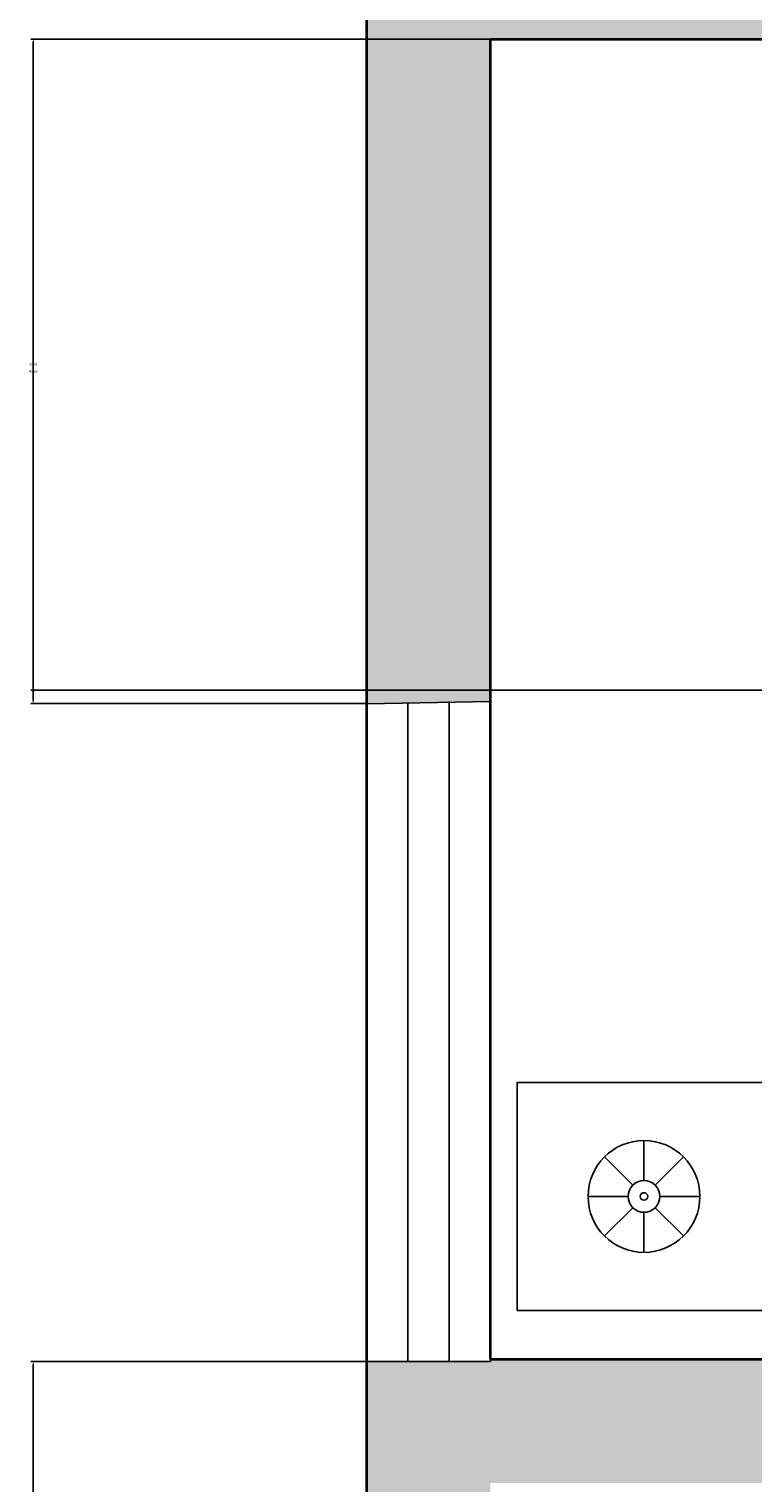
# Model space of a CAD drawing. Units: millimetres. Extents: x 2817 to 5038, y 1110 to 3565.
# Tile 2 of 21: x 2817 to 2870, y 1265 to 1371. Entities that reach past the tile are written whole.
import ezdxf

# ---------------------------------------------------------------- set-up
doc = ezdxf.new("R2010")
doc.units = ezdxf.units.MM
for name, color, linetype, lineweight in [('A-ANNO-DIMS', 2, 'Continuous', 18), ('A-WALL', 7, 'Continuous', 35), ('DOOR&WINDOW', 1, 'Continuous', 25), ('FURNITURE', 219, 'Continuous', 18)]:
    doc.layers.add(name, color=color, linetype=linetype, lineweight=lineweight)
doc.layers.add('A-WALL-PATT', color=51, linetype='Continuous', lineweight=13, true_color=0xf7f281)
doc.layers.add('BLOCK', color=6, linetype='Continuous')
doc.styles.get("Standard").update_dxf_attribs({"font": 'arial.ttf'})
doc.dimstyles.get("Standard").update_dxf_attribs({"dimtxt": 0.18, "dimasz": 0.18, "dimexe": 0.18, "dimexo": 0.0625, "dimgap": 0.09, "dimtad": 0, "dimtih": 1, "dimtoh": 1, "dimdec": 4, "dimzin": 0, "dimdsep": 46, "dimtxsty": 'Standard', "dimcen": 0.09, "dimadec": 0, "dimazin": 0, "dimtfac": 1, "dimtdec": 4, "dimtofl": 0, "dimtmove": 0, "dimatfit": 3, "dimfxl": 1, "dimtolj": 1, "dimtzin": 0, "dimarcsym": 0})

# ---------------------------------------------------------------- blocks, each defined once
blk = doc.blocks.new('A$C52E67D0D')
at = {"layer": 'BLOCK'}
for p, q in [((2251.5, 1605.5), (2251.5, 1684.7)), ((2229.3, 1596.3), (2173.3, 1652.3)), ((2273.7, 1596.3), (2329.7, 1652.3)), ((2220.1, 1574.1), (2140.9, 1574.1)), ((2282.9, 1574.1), (2362.1, 1574.1)), ((2229.3, 1551.9), (2173.3, 1495.9)), ((2251.5, 1542.8), (2251.5, 1463.5)), ((2273.7, 1551.9), (2329.7, 1495.9))]:
    blk.add_line(p, q, dxfattribs=at)
blk.add_lwpolyline([(2001, 1348.6), (2001, 1799.6), (2502, 1799.6), (2502, 1348.6)], close=True, dxfattribs=at)
for radius in [110.6, 31.4, 7.46]:
    blk.add_circle((2251.5, 1574.1), radius, dxfattribs=at)
blk = doc.blocks.new('WIN-4FT')
for p, q in [((0, 47.85), (9, 48)), ((0, 0), (0, 47.85)), ((3, 0), (3, 47.85)), ((6, 48), (6, 0)), ((9, 48), (9, 0)), ((9, 0), (0, 0))]:
    blk.add_line(p, q)
blk = doc.blocks.new('*D31')
at = {"layer": 'A-ANNO-DIMS', "color": 0, "lineweight": -2, "transparency": 16777216}
for p, q in [((2841.68, 1274.26), (2817.31, 1274.26)), ((2817.49, 1274.08), (2817.49, 1233.89)), ((2817.49, 1193.33), (2817.49, 1233.52)), ((2841.68, 1193.15), (2817.31, 1193.15))]:
    blk.add_line(p, q, dxfattribs=at)
for points in [[(2817.46, 1274.08), (2817.52, 1274.08), (2817.49, 1274.26)], [(2817.46, 1193.33), (2817.52, 1193.33), (2817.49, 1193.15)]]:
    blk.add_solid(points, dxfattribs=at)
at = {"layer": 'Defpoints', "color": 0, "lineweight": -2, "transparency": 16777216}
for p in [(2817.49, 1274.26), (2841.74, 1274.26), (2841.74, 1193.15)]:
    blk.add_point(p, dxfattribs=at)
at = {"layer": 'A-ANNO-DIMS', "color": 0, "transparency": 16777216, "insert": (2817.49, 1233.7), "char_height": 0.18, "attachment_point": 5}
blk.add_mtext('\\A1;81.1', dxfattribs=at)
blk = doc.blocks.new('*D32')
at = {"layer": 'A-ANNO-DIMS', "color": 0, "lineweight": -2, "transparency": 16777216}
for p, q in [((2850.68, 1370.44), (2817.31, 1370.44)), ((2817.49, 1370.26), (2817.49, 1346.45)), ((2817.49, 1322.29), (2817.49, 1346.09)), ((2841.68, 1322.11), (2817.31, 1322.11))]:
    blk.add_line(p, q, dxfattribs=at)
for points in [[(2817.46, 1370.26), (2817.52, 1370.26), (2817.49, 1370.44)], [(2817.46, 1322.29), (2817.52, 1322.29), (2817.49, 1322.11)]]:
    blk.add_solid(points, dxfattribs=at)
at = {"layer": 'Defpoints', "color": 0, "lineweight": -2, "transparency": 16777216}
for p in [(2817.49, 1370.44), (2850.74, 1370.44), (2841.74, 1322.11)]:
    blk.add_point(p, dxfattribs=at)
at = {"layer": 'A-ANNO-DIMS', "color": 0, "transparency": 16777216, "insert": (2817.49, 1346.27), "char_height": 0.18, "attachment_point": 5}
blk.add_mtext('\\A1;48.33', dxfattribs=at)
blk = doc.blocks.new('*D47')
at = {"layer": 'A-ANNO-DIMS', "color": 0, "lineweight": -2, "transparency": 16777216}
for p, q in [((3052.18, 1370.44), (2817.31, 1370.44)), ((2817.49, 1370.26), (2817.49, 1346.95)), ((2817.49, 1323.28), (2817.49, 1346.58)), ((3052.08, 1323.1), (2817.31, 1323.1))]:
    blk.add_line(p, q, dxfattribs=at)
for points in [[(2817.46, 1370.26), (2817.52, 1370.26), (2817.49, 1370.44)], [(2817.46, 1323.28), (2817.52, 1323.28), (2817.49, 1323.1)]]:
    blk.add_solid(points, dxfattribs=at)
at = {"layer": 'Defpoints', "color": 0, "lineweight": -2, "transparency": 16777216}
for p in [(2817.49, 1370.44), (3052.24, 1370.44), (3052.14, 1323.1)]:
    blk.add_point(p, dxfattribs=at)
at = {"layer": 'A-ANNO-DIMS', "color": 0, "transparency": 16777216, "insert": (2817.49, 1346.77), "char_height": 0.18, "attachment_point": 5}
blk.add_mtext('\\A1;47.34', dxfattribs=at)

msp = doc.modelspace()

# ---------------------------------------------------------------- hatches: boundary and pattern name
at = {"layer": 'A-WALL-PATT'}
h = msp.add_hatch(color=256, dxfattribs=at)
h.dxf.hatch_style = 1
h.paths.add_polyline_path([(3186.7393, 1614.4357), (2841.7393, 1614.4357), (2841.7393, 1568.614), (2850.7393, 1568.7609), (2850.7393, 1605.4357), (2982.7393, 1605.4357), (2991.7393, 1605.4357), (3052.2393, 1605.4357), (3052.2393, 1573.7835), (3061.2393, 1573.7835), (3061.2393, 1605.4357), (3182.2393, 1605.4357), (3182.2393, 1143.4357), (3181.2393, 1143.4357), (3181.2393, 1134.4357), (3186.7393, 1134.4357)])
h.paths.add_polyline_path([(3061.2393, 1143.4357), (3061.2393, 1147.4357), (3052.2393, 1147.4357), (3052.2393, 1143.4357), (2850.7393, 1143.4357), (2850.7393, 1145.2996), (2841.7393, 1145.2996), (2841.7393, 1134.4357), (3061.2393, 1134.4357)], flags=17)
h.paths.add_polyline_path([(2850.7393, 1265.4357), (2946.7393, 1265.4357), (2946.7393, 1270.8357), (2946.7393, 1274.4357), (2850.7393, 1274.4357), (2850.7381, 1274.4357), (2850.7381, 1274.2564), (2841.7393, 1274.2564), (2841.7393, 1193.1527), (2850.7393, 1193.2996)], flags=17)
h.paths.add_polyline_path([(3061.2393, 1299.098), (3052.2393, 1299.098), (3052.2393, 1274.4357), (2991.7393, 1274.4357), (2991.7393, 1340.4357), (2982.7393, 1340.4357), (2982.7393, 1274.4357), (2982.7393, 1265.4357), (3052.2393, 1265.4357), (3052.2393, 1259.143), (3061.2393, 1259.2899)], flags=17)
h.paths.add_polyline_path([(3061.2393, 1383.4357), (3052.2393, 1383.4357), (3052.2393, 1379.4357), (2931.7393, 1379.4357), (2922.7393, 1379.4357), (2850.7393, 1379.4357), (2850.7381, 1379.4357), (2850.7381, 1379.3646), (2841.7393, 1379.3646), (2841.7393, 1322.1095), (2850.7393, 1322.2564), (2850.7393, 1370.4357), (2982.7393, 1370.4357), (2987.2393, 1370.4357), (3017.2393, 1370.4357), (3052.2393, 1370.4357), (3052.2393, 1323.098), (3061.2393, 1323.098)], flags=17)

# ---------------------------------------------------------------- linework, layer by layer
at = {"layer": 'A-WALL'}
for p, q in [((2841.7393, 1134.4357), (2841.7393, 1614.4357)), ((2850.7393, 1370.4357), (2982.7393, 1370.4357)), ((2850.7393, 1274.4357), (2850.7393, 1370.4357)), ((2850.7393, 1274.4357), (2946.7393, 1274.4357))]:
    msp.add_line(p, q, dxfattribs=at)

# ---------------------------------------------------------------- block references
at = {"layer": 'DOOR&WINDOW'}
msp.add_blockref('WIN-4FT', (2841.7381, 1274.2563), dxfattribs=at)
at = {"layer": 'FURNITURE', "xscale": 0.0367705835331598, "yscale": 0.0367705835331598, "zscale": 0.0367705835331598, "rotation": 180}
msp.add_blockref('A$C52E67D0D', (2944.6948, 1344.1495), dxfattribs=at)

# ---------------------------------------------------------------- dimensions: what is measured, and where the dimension line sits
at = {"layer": 'A-ANNO-DIMS'}
for base, p1, p2, override, picture, middle in [((2817.4881, 1370.4357), (2841.7393, 1322.1095), (2850.7393, 1370.4357), {"dimdec": 2, "dimlfac": 1, "dimrnd": 0, "dimzin": 0, "dimdsep": 46, "dimlunit": 2}, '*D32', (2817.4881, 1346.2726)), ((2817.4881, 1370.4357), (3052.1378, 1323.098), (3052.2393, 1370.4357), {"dimdec": 2, "dimlfac": 1, "dimrnd": 0, "dimzin": 0, "dimdsep": 46, "dimlunit": 2}, '*D47', (2817.4881, 1346.7669)), ((2817.4881, 1274.2564), (2841.7405, 1193.1527), (2841.7381, 1274.2564), {"dimdec": 1, "dimlfac": 1, "dimrnd": 0, "dimzin": 0, "dimdsep": 46, "dimlunit": 2}, '*D31', (2817.4881, 1233.7046))]:
    dim = msp.add_linear_dim(base=base, p1=p1, p2=p2, angle=90, dimstyle='Standard', override=override, dxfattribs=at)
    dim.commit()
    dim.dimension.update_dxf_attribs({"geometry": picture, "text_midpoint": middle})

doc.saveas('drawing.dxf')
